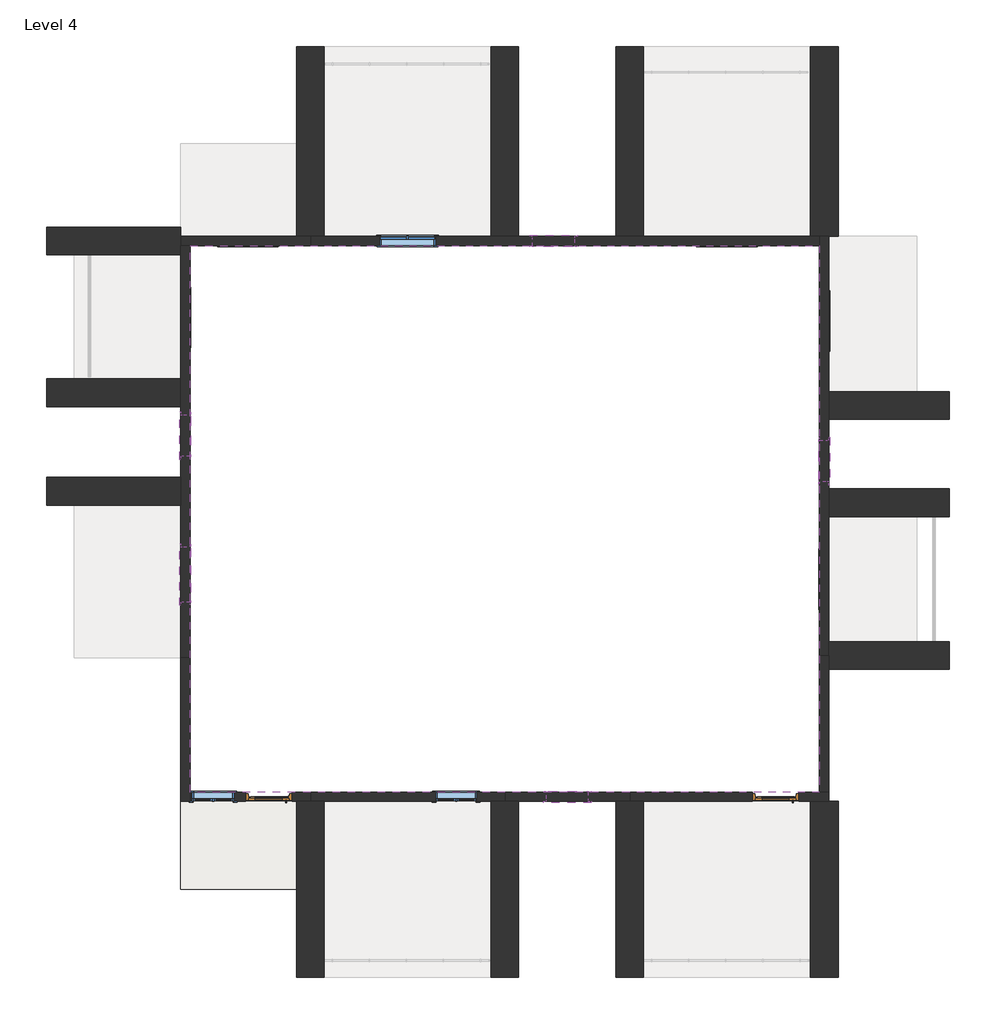
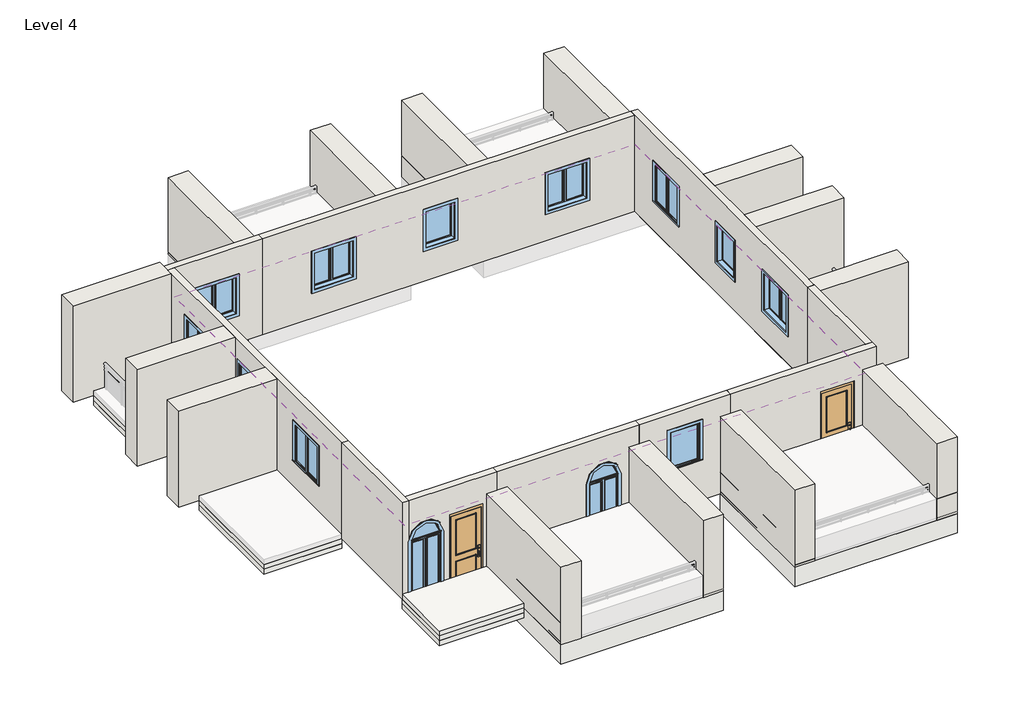
# One storey, part 1 of 2: 24 walls, 13 windows, 5 slabs, 2 doors, 1 covering.
"""IFC4 building model written with IfcOpenShell, lengths in millimetres."""

from ifc_helpers import new_model, si_unit, frame, origin, place, context, project, spatial, polyline, circle_curve, outline, extrude, faceted_brep, transform, mapped, element, save
from ifc_brep_helpers import plane_surface, revolved_surface, advanced_brep
from components import door_b6c2ee01, window_4e95f2a8, window_0862ab64, window_3a1167bf, window_8a4441b2

model = new_model("IFC4")

# Units and contexts
model_context = context("Model", 3, world=origin())
ifc_project = project(units=[si_unit("LENGTHUNIT", "METRE", prefix="MILLI")], contexts=[model_context])

# Site, building, storey
site = spatial("IfcSite", under=ifc_project)
building = spatial("IfcBuilding", under=site)
storey = spatial("IfcBuildingStorey", under=building, Name="Level 4", Elevation=9144.0)

# Covering
placement = place(None, origin())
element("IfcCovering", 1, ObjectType="2' x 4' ACT System", at=placement, inside=storey, context=model_context, shape_type="SweptSolid", body=[
    extrude(outline(polyline([(-12179.4937431, 6319.013611), (-9537.8937431, 6319.013611), (1638.1062569, 6319.013611), (1638.1062569, -2672.586389), (1638.1062569, -5669.786389), (-2527.4937431, -5669.786389), (-5270.6937431, -5669.786389), (-9537.8937431, -5669.786389), (-12179.4937431, -5669.786389), (-12179.4937431, -2723.386389), (-12179.4937431, 6319.013611)])), frame((0.0, 0.0, 11582.4), z_axis=(0.0, 0.0, 1.0), x_axis=(1.0, 0.0, 0.0)), (0.0, 0.0, 1.0), 57.15),
])

# Doors
door_shape = door_b6c2ee01(model_context)
element("IfcDoor", 2, ObjectType="Door-Exterior-Single-Two_Lite : 36\" x 94\"", at=placement, inside=storey, context=model_context, shape_type="MappedRepresentation", body=[
    mapped(door_shape, transform((-10452.2937431, -5765.036389, 9144.0), x_axis=(-1.0, 0.0, 0.0), y_axis=(0.0, -1.0, 0.0), z_axis=(0.0, 0.0, 1.0))),
])
element("IfcDoor", 3, ObjectType="Door-Exterior-Single-Two_Lite : 36\" x 94\"", at=placement, inside=storey, context=model_context, shape_type="MappedRepresentation", body=[
    mapped(door_shape, transform((672.9062569, -5765.036389, 9144.0), x_axis=(-1.0, 0.0, 0.0), y_axis=(0.0, -1.0, 0.0), z_axis=(0.0, 0.0, 1.0))),
])

# Slabs
element("IfcSlab", 4, ObjectType="Generic - 2' 2", at=placement, inside=storey, context=model_context, shape_type="SweptSolid", body=[
    extrude(outline(polyline([(-4965.8937431, -9733.786389), (-9842.6937431, -9733.786389), (-9842.6937431, -5872.986389), (-4965.8937431, -5872.986389), (-4965.8937431, -9733.786389)])), frame((0.0, 0.0, 8839.2), z_axis=(0.0, 0.0, 1.0), x_axis=(1.0, 0.0, 0.0)), (0.0, 0.0, 1.0), 609.6),
])
element("IfcSlab", 5, ObjectType="Generic - 2' 2", at=placement, inside=storey, context=model_context, shape_type="SweptSolid", body=[
    extrude(outline(polyline([(2044.5062569, -9733.786389), (-2832.2937431, -9733.786389), (-2832.2937431, -5872.986389), (2044.5062569, -5872.986389), (2044.5062569, -9733.786389)])), frame((0.0, 0.0, 8839.2), z_axis=(0.0, 0.0, 1.0), x_axis=(1.0, 0.0, 0.0)), (0.0, 0.0, 1.0), 609.6),
])
element("IfcSlab", 6, ObjectType="general 6\"", at=placement, inside=storey, context=model_context, shape_type="SweptSolid", body=[
    extrude(outline(polyline([(-14722.8064179, 6115.813611), (-12382.6937431, 6115.813611), (-12382.6937431, 3398.013611), (-14722.8064179, 3398.013611), (-14722.8064179, 6115.813611)])), frame((0.0, 0.0, 9144.0), z_axis=(0.0, 0.0, 1.0), x_axis=(1.0, 0.0, 0.0)), (0.0, 0.0, 1.0), 152.4),
    extrude(outline(polyline([(-14722.8064179, 629.413611), (-12382.6937431, 629.413611), (-12382.6937431, -2723.386389), (-14722.8064179, -2723.386389), (-14722.8064179, 629.413611)])), frame((0.0, 0.0, 9144.0), z_axis=(0.0, 0.0, 1.0), x_axis=(1.0, 0.0, 0.0)), (0.0, 0.0, 1.0), 152.4),
    extrude(outline(polyline([(-9842.6937431, -5872.986389), (-9842.6937431, -7803.386389), (-12382.6937431, -7803.386389), (-12382.6937431, -5872.986389), (-9842.6937431, -5872.986389)])), frame((0.0, 0.0, 9144.0), z_axis=(0.0, 0.0, 1.0), x_axis=(1.0, 0.0, 0.0)), (0.0, 0.0, 1.0), 152.4),
    extrude(outline(polyline([(3771.7062569, -2367.786389), (1841.3062569, -2367.786389), (1841.3062569, 426.213611), (3771.7062569, 426.213611), (3771.7062569, -2367.786389)])), frame((0.0, 0.0, 9144.0), z_axis=(0.0, 0.0, 1.0), x_axis=(1.0, 0.0, 0.0)), (0.0, 0.0, 1.0), 152.4),
    extrude(outline(polyline([(3771.7062569, 3118.613611), (1841.3062569, 3118.613611), (1841.3062569, 6522.213611), (3771.7062569, 6522.213611), (3771.7062569, 3118.613611)])), frame((0.0, 0.0, 9144.0), z_axis=(0.0, 0.0, 1.0), x_axis=(1.0, 0.0, 0.0)), (0.0, 0.0, 1.0), 152.4),
    extrude(outline(polyline([(-12382.6937431, 6522.213611), (-12382.6937431, 8557.6995084), (-9842.6937431, 8557.6995084), (-9842.6937431, 6522.213611), (-12382.6937431, 6522.213611)])), frame((0.0, 0.0, 9144.0), z_axis=(0.0, 0.0, 1.0), x_axis=(1.0, 0.0, 0.0)), (0.0, 0.0, 1.0), 152.4),
])
element("IfcSlab", 7, ObjectType="general 6\" 2", at=placement, inside=storey, context=model_context, shape_type="SweptSolid", body=[
    extrude(outline(polyline([(3771.7062569, -2367.786389), (1841.3062569, -2367.786389), (1841.3062569, 375.413611), (3771.7062569, 375.413611), (3771.7062569, -2367.786389)])), frame((0.0, 0.0, 9296.4), z_axis=(0.0, 0.0, 1.0), x_axis=(1.0, 0.0, 0.0)), (0.0, 0.0, 1.0), 152.4),
    extrude(outline(polyline([(3771.7062569, 3118.613611), (1841.3062569, 3118.613611), (1841.3062569, 6522.213611), (3771.7062569, 6522.213611), (3771.7062569, 3118.613611)])), frame((0.0, 0.0, 9296.4), z_axis=(0.0, 0.0, 1.0), x_axis=(1.0, 0.0, 0.0)), (0.0, 0.0, 1.0), 152.4),
    extrude(outline(polyline([(-12382.6937431, 6522.213611), (-12382.6937431, 8557.6995084), (-9842.6937431, 8557.6995084), (-9842.6937431, 6522.213611), (-12382.6937431, 6522.213611)])), frame((0.0, 0.0, 9296.4), z_axis=(0.0, 0.0, 1.0), x_axis=(1.0, 0.0, 0.0)), (0.0, 0.0, 1.0), 152.4),
    extrude(outline(polyline([(-14722.8064179, 6115.813611), (-12384.3500805, 6115.813611), (-12384.3500805, 3398.013611), (-14722.8064179, 3398.013611), (-14722.8064179, 6115.813611)])), frame((0.0, 0.0, 9296.4), z_axis=(0.0, 0.0, 1.0), x_axis=(1.0, 0.0, 0.0)), (0.0, 0.0, 1.0), 152.4),
    extrude(outline(polyline([(-14722.8064179, -2723.386389), (-14722.8064179, 629.413611), (-12382.6937431, 629.413611), (-12382.6937431, -2723.386389), (-14722.8064179, -2723.386389)])), frame((0.0, 0.0, 9296.4), z_axis=(0.0, 0.0, 1.0), x_axis=(1.0, 0.0, 0.0)), (0.0, 0.0, 1.0), 152.4),
    extrude(outline(polyline([(-9842.6937431, -5872.986389), (-9842.6937431, -7803.386389), (-12382.6937431, -7803.386389), (-12382.6937431, -5872.986389), (-9842.6937431, -5872.986389)])), frame((0.0, 0.0, 9296.4), z_axis=(0.0, 0.0, 1.0), x_axis=(1.0, 0.0, 0.0)), (0.0, 0.0, 1.0), 152.4),
])
element("IfcSlab", 8, ObjectType="general 6\" 3", at=placement, inside=storey, context=model_context, shape_type="SweptSolid", body=[
    extrude(outline(polyline([(-12382.6937431, -5872.986389), (-9842.6937431, -5872.986389), (-9842.6937431, -7803.386389), (-12382.6937431, -7803.386389), (-12382.6937431, -5872.986389)])), frame((0.0, 0.0, 9448.8), z_axis=(0.0, 0.0, 1.0), x_axis=(1.0, 0.0, 0.0)), (0.0, 0.0, 1.0), 152.4),
])

# Walls
element("IfcWall", 9, ObjectType="Generic - 8\"", at=placement, inside=storey, context=model_context, shape_type="Brep", body=[
    faceted_brep([(-12382.6937431, 6319.013611, 9448.8), (-12179.4937431, 6319.013611, 9448.8), (-9537.8937431, 6319.013611, 9448.8), (-9537.8937431, 6319.013611, 12496.8), (-12179.4937431, 6319.013611, 12496.8), (-12382.6937431, 6319.013611, 12496.8), (-10299.8937431, 6319.013611, 11582.4), (-10299.8937431, 6319.013611, 10363.2), (-11519.0937431, 6319.013611, 10363.2), (-11519.0937431, 6319.013611, 11582.4), (-12382.6937431, 6522.213611, 9448.8), (-12382.6937431, 6522.213611, 12496.8), (-9537.8937431, 6522.213611, 12496.8), (-9537.8937431, 6522.213611, 9448.8), (-9842.6937431, 6522.213611, 9448.8), (-10299.8937431, 6522.213611, 11582.4), (-11519.0937431, 6522.213611, 11582.4), (-11519.0937431, 6522.213611, 10363.2), (-10299.8937431, 6522.213611, 10363.2)], [[[0, 1, 2, 3, 4, 5], [6, 7, 8, 9]], [[10, 11, 12, 13, 14], [15, 16, 17, 18]], [[2, 1, 0, 10, 14, 13]], [[5, 4, 3, 12, 11]], [[0, 5, 11, 10]], [[7, 6, 15, 18]], [[8, 7, 18, 17]], [[9, 8, 17, 16]], [[6, 9, 16, 15]], [[2, 13, 12, 3]]]),
])
element("IfcWall", 10, ObjectType="Generic - 8\"", at=placement, inside=storey, context=model_context, shape_type="Brep", body=[
    faceted_brep([(-12179.4937431, -5872.986389, 9448.8), (-12179.4937431, -5669.786389, 9448.8), (-12179.4937431, -2723.386389, 9448.8), (-12179.4937431, -2723.386389, 12496.8), (-12179.4937431, -5669.786389, 12496.8), (-12179.4937431, -5872.986389, 12496.8), (-12382.6937431, -5872.986389, 9448.8), (-12382.6937431, -5872.986389, 12496.8), (-12382.6937431, -2723.386389, 12496.8), (-12382.6937431, -2723.386389, 9448.8)], [[[0, 1, 2, 3, 4, 5]], [[6, 7, 8, 9]], [[2, 1, 0, 6, 9]], [[3, 2, 9, 8]], [[5, 4, 3, 8, 7]], [[0, 5, 7, 6]]]),
])
element("IfcWall", 11, ObjectType="Generic - 8\"", at=placement, inside=storey, context=model_context, shape_type="Brep", body=[
    faceted_brep([(-2527.4937431, -5669.786389, 12496.8), (1638.1062569, -5669.786389, 12496.8), (1841.3062569, -5669.786389, 12496.8), (1841.3062569, -5669.786389, 9448.8), (1638.1062569, -5669.786389, 9448.8), (1180.9062569, -5669.786389, 9448.8), (1180.9062569, -5669.786389, 11633.2), (164.9062569, -5669.786389, 11633.2), (164.9062569, -5669.786389, 9448.8), (-2527.4937431, -5669.786389, 9448.8), (1841.3062569, -5872.986389, 12496.8), (-2527.4937431, -5872.986389, 12496.8), (-2527.4937431, -5872.986389, 9448.8), (-2222.6937431, -5872.986389, 9448.8), (164.9062569, -5872.986389, 9448.8), (164.9062569, -5872.986389, 11633.2), (1180.9062569, -5872.986389, 11633.2), (1180.9062569, -5872.986389, 9448.8), (1434.9062569, -5872.986389, 9448.8), (1841.3062569, -5872.986389, 9448.8)], [[[0, 1, 2, 3, 4, 5, 6, 7, 8, 9]], [[10, 11, 12, 13, 14, 15, 16, 17, 18, 19]], [[3, 19, 18, 17, 5, 4]], [[12, 9, 8, 14, 13]], [[2, 1, 0, 11, 10]], [[2, 10, 19, 3]], [[7, 15, 14, 8]], [[15, 7, 6, 16]], [[16, 6, 5, 17]], [[9, 12, 11, 0]]]),
])
element("IfcWall", 12, ObjectType="Generic - 8\"", at=placement, inside=storey, context=model_context, shape_type="Brep", body=[
    faceted_brep([(1638.1062569, 6522.213611, 12496.8), (1638.1062569, 6522.213611, 9448.8), (1638.1062569, 6319.013611, 9448.8), (1638.1062569, -2672.586389, 9448.8), (1638.1062569, -2672.586389, 12496.8), (1638.1062569, 6319.013611, 12496.8), (1638.1062569, 1137.413611, 11653.6747769), (1638.1062569, 1137.413611, 10434.4747769), (1638.1062569, 2051.813611, 10434.4747769), (1638.1062569, 2051.813611, 11653.6747769), (1638.1062569, -1605.786389, 11593.5712595), (1638.1062569, -1605.786389, 10374.3712595), (1638.1062569, -386.586389, 10374.3712595), (1638.1062569, -386.586389, 11593.5712595), (1638.1062569, 4058.413611, 11593.5712595), (1638.1062569, 4058.413611, 10374.3712595), (1638.1062569, 5277.613611, 10374.3712595), (1638.1062569, 5277.613611, 11593.5712595), (1841.3062569, 6522.213611, 9448.8), (1841.3062569, 6522.213611, 12496.8), (1841.3062569, 3118.613611, 12496.8), (1841.3062569, 2509.013611, 12496.8), (1841.3062569, 985.013611, 12496.8), (1841.3062569, 375.413611, 12496.8), (1841.3062569, -2367.786389, 12496.8), (1841.3062569, -2672.586389, 12496.8), (1841.3062569, -2672.586389, 9448.8), (1841.3062569, -2367.786389, 9448.8), (1841.3062569, 375.413611, 9448.8), (1841.3062569, 985.013611, 9448.8), (1841.3062569, 2509.013611, 9448.8), (1841.3062569, 3118.613611, 9448.8), (1841.3062569, 1137.413611, 11653.6747769), (1841.3062569, 2051.813611, 11653.6747769), (1841.3062569, 2051.813611, 10434.4747769), (1841.3062569, 1137.413611, 10434.4747769), (1841.3062569, -1605.786389, 11593.5712595), (1841.3062569, -386.586389, 11593.5712595), (1841.3062569, -386.586389, 10374.3712595), (1841.3062569, -1605.786389, 10374.3712595), (1841.3062569, 4058.413611, 11593.5712595), (1841.3062569, 5277.613611, 11593.5712595), (1841.3062569, 5277.613611, 10374.3712595), (1841.3062569, 4058.413611, 10374.3712595)], [[[0, 1, 2, 3, 4, 5], [6, 7, 8, 9], [10, 11, 12, 13], [14, 15, 16, 17]], [[18, 19, 20, 21, 22, 23, 24, 25, 26, 27, 28, 29, 30, 31], [32, 33, 34, 35], [36, 37, 38, 39], [40, 41, 42, 43]], [[3, 2, 1, 18, 31, 30, 29, 28, 27, 26]], [[4, 3, 26, 25]], [[0, 5, 4, 25, 24, 23, 22, 21, 20, 19]], [[0, 19, 18, 1]], [[7, 6, 32, 35]], [[8, 7, 35, 34]], [[9, 8, 34, 33]], [[6, 9, 33, 32]], [[11, 10, 36, 39]], [[12, 11, 39, 38]], [[13, 12, 38, 37]], [[10, 13, 37, 36]], [[15, 14, 40, 43]], [[16, 15, 43, 42]], [[17, 16, 42, 41]], [[14, 17, 41, 40]]]),
])
element("IfcWall", 13, ObjectType="Generic - 8\"", at=placement, inside=storey, context=model_context, shape_type="Brep", body=[
    faceted_brep([(-12179.4937431, -2723.386389, 9448.8), (-12179.4937431, 6319.013611, 9448.8), (-12179.4937431, 6319.013611, 12496.8), (-12179.4937431, -2723.386389, 12496.8), (-12179.4937431, 2610.613611, 11819.7149116), (-12179.4937431, 2610.613611, 10600.5149116), (-12179.4937431, 1696.213611, 10600.5149116), (-12179.4937431, 1696.213611, 11819.7149116), (-12179.4937431, -284.986389, 11642.8059909), (-12179.4937431, -284.986389, 10423.6059909), (-12179.4937431, -1504.186389, 10423.6059909), (-12179.4937431, -1504.186389, 11642.8059909), (-12179.4937431, 5353.813611, 11569.1335827), (-12179.4937431, 5353.813611, 10349.9335827), (-12179.4937431, 4134.613611, 10349.9335827), (-12179.4937431, 4134.613611, 11569.1335827), (-12382.6937431, -2723.386389, 9448.8), (-12382.6937431, -2723.386389, 12496.8), (-12382.6937431, 629.413611, 12496.8), (-12382.6937431, 1239.013611, 12496.8), (-12382.6937431, 2788.413611, 12496.8), (-12382.6937431, 3398.013611, 12496.8), (-12382.6937431, 6115.813611, 12496.8), (-12382.6937431, 6319.013611, 12496.8), (-12382.6937431, 6319.013611, 9448.8), (-12382.6937431, 6115.813611, 9448.8), (-12382.6937431, 3398.013611, 9448.8), (-12382.6937431, 2788.413611, 9448.8), (-12382.6937431, 1239.013611, 9448.8), (-12382.6937431, 629.413611, 9448.8), (-12382.6937431, 2610.613611, 11819.7149116), (-12382.6937431, 1696.213611, 11819.7149116), (-12382.6937431, 1696.213611, 10600.5149116), (-12382.6937431, 2610.613611, 10600.5149116), (-12382.6937431, -284.986389, 11642.8059909), (-12382.6937431, -1504.186389, 11642.8059909), (-12382.6937431, -1504.186389, 10423.6059909), (-12382.6937431, -284.986389, 10423.6059909), (-12382.6937431, 5353.813611, 11569.1335827), (-12382.6937431, 4134.613611, 11569.1335827), (-12382.6937431, 4134.613611, 10349.9335827), (-12382.6937431, 5353.813611, 10349.9335827)], [[[0, 1, 2, 3], [4, 5, 6, 7], [8, 9, 10, 11], [12, 13, 14, 15]], [[16, 17, 18, 19, 20, 21, 22, 23, 24, 25, 26, 27, 28, 29], [30, 31, 32, 33], [34, 35, 36, 37], [38, 39, 40, 41]], [[1, 0, 16, 29, 28, 27, 26, 25, 24]], [[3, 2, 23, 22, 21, 20, 19, 18, 17]], [[0, 3, 17, 16]], [[2, 1, 24, 23]], [[5, 4, 30, 33]], [[6, 5, 33, 32]], [[7, 6, 32, 31]], [[4, 7, 31, 30]], [[9, 8, 34, 37]], [[10, 9, 37, 36]], [[11, 10, 36, 35]], [[8, 11, 35, 34]], [[13, 12, 38, 41]], [[14, 13, 41, 40]], [[15, 14, 40, 39]], [[12, 15, 39, 38]]]),
])
element("IfcWall", 14, ObjectType="Generic - 8\"", at=placement, inside=storey, context=model_context, shape_type="AdvancedBrep", body=[
    advanced_brep(
    [(-12179.4937431, -5669.786389, 12496.8), (-9537.8937431, -5669.786389, 12496.8), (-9537.8937431, -5669.786389, 9448.8), (-9944.2937431, -5669.786389, 9448.8), (-9944.2937431, -5669.786389, 11633.2), (-10960.2937431, -5669.786389, 11633.2), (-10960.2937431, -5669.786389, 9448.8), (-11214.2937431, -5669.786389, 9448.8), (-11214.2937431, -5669.786389, 11187.597687), (-12128.6937431, -5669.786389, 11187.597687), (-12128.6937431, -5669.786389, 9448.8), (-12179.4937431, -5669.786389, 9448.8), (-9537.8937431, -5872.986389, 12496.8), (-12179.4937431, -5872.986389, 12496.8), (-12179.4937431, -5872.986389, 9448.8), (-12128.6937431, -5872.986389, 9448.8), (-12128.6937431, -5872.986389, 11187.597687), (-11214.2937431, -5872.986389, 11187.597687), (-11214.2937431, -5872.986389, 9448.8), (-10960.2937431, -5872.986389, 9448.8), (-10960.2937431, -5872.986389, 11633.2), (-9944.2937431, -5872.986389, 11633.2), (-9944.2937431, -5872.986389, 9448.8), (-9842.6937431, -5872.986389, 9448.8), (-9537.8937431, -5872.986389, 9448.8)],
    [
        (0, 1),
        (1, 2),
        (2, 3),
        (3, 4),
        (4, 5),
        (5, 6),
        (6, 7),
        (7, 8),
        (8, 9, circle_curve(frame((-11671.4937431, -5669.786389, 11187.597687), z_axis=(0.0, -1.0, 0.0), x_axis=(-1.0, 0.0, 0.0)), 457.2)),
        (9, 10),
        (10, 11),
        (11, 0),
        (12, 13),
        (13, 14),
        (14, 15),
        (15, 16),
        (16, 17, circle_curve(frame((-11671.4937431, -5872.986389, 11187.597687), z_axis=(0.0, 1.0, 0.0), x_axis=(-1.0, 0.0, 0.0)), 457.2)),
        (17, 18),
        (18, 19),
        (19, 20),
        (20, 21),
        (21, 22),
        (22, 23),
        (23, 24),
        (24, 12),
        (14, 11),
        (10, 15),
        (2, 24),
        (22, 3),
        (6, 19),
        (18, 7),
        (0, 13),
        (12, 1),
        (5, 20),
        (4, 21),
        (9, 16),
        (17, 8),
    ],
    [
        plane_surface(frame((1423.3958892, -5669.786389, 9448.8), z_axis=(0.0, 1.0, 0.0), x_axis=(-1.0, 0.0, 0.0))),
        plane_surface(frame((1423.3958892, -5872.986389, 9448.8), z_axis=(0.0, -1.0, 0.0), x_axis=(1.0, 0.0, 0.0))),
        plane_surface(frame((-9537.8937431, -5669.786389, 9448.8), z_axis=(0.0, 0.0, -1.0), x_axis=(0.0, -1.0, 0.0))),
        plane_surface(frame((-12281.0937431, -5669.786389, 12496.8), z_axis=(0.0, 0.0, 1.0), x_axis=(0.0, -1.0, 0.0))),
        plane_surface(frame((-12179.4937431, 6416.9740134, 9448.8), z_axis=(-1.0, 0.0, 0.0), x_axis=(0.0, 1.0, 0.0))),
        plane_surface(frame((-9537.8937431, -5669.786389, 12496.8), z_axis=(1.0, 0.0, 0.0), x_axis=(0.0, -1.0, 0.0))),
        plane_surface(frame((-10960.2937431, -4145.786389, 9144.0), z_axis=(1.0, 0.0, 0.0), x_axis=(0.0, -1.0, 0.0))),
        plane_surface(frame((-10960.2937431, -4145.786389, 11633.2), z_axis=(0.0, 0.0, -1.0), x_axis=(0.0, -1.0, 0.0))),
        plane_surface(frame((-9944.2937431, -4145.786389, 11633.2), z_axis=(-1.0, 0.0, 0.0), x_axis=(0.0, -1.0, 0.0))),
        plane_surface(frame((-12128.6937431, -7193.786389, 11187.597687), z_axis=(1.0, 0.0, 0.0), x_axis=(0.0, 1.0, 0.0))),
        plane_surface(frame((-11214.2937431, -7193.786389, 9339.747687), z_axis=(-1.0, 0.0, 0.0), x_axis=(0.0, 1.0, 0.0))),
        revolved_surface(polyline([(-12128.6937431, -5872.986389, 11187.597687), (-12128.6937431, -5669.786389, 11187.597687)]), (-11671.4937431, -4145.786389, 11187.597687), (0.0, -1.0, 0.0)),
    ],
    [
        (0, [[1, 2, 3, 4, 5, 6, 7, 8, 9, 10, 11, 12]]),
        (1, [[13, 14, 15, 16, 17, 18, 19, 20, 21, 22, 23, 24, 25]]),
        (2, [[26, -11, 27, -15]]),
        (2, [[28, -24, -23, 29, -3]]),
        (2, [[30, -19, 31, -7]]),
        (3, [[-1, 32, -13, 33]]),
        (4, [[-12, -26, -14, -32]]),
        (5, [[-33, -25, -28, -2]]),
        (6, [[34, -20, -30, -6]]),
        (7, [[-34, -5, 35, -21]]),
        (8, [[-35, -4, -29, -22]]),
        (9, [[36, -16, -27, -10]]),
        (10, [[37, -8, -31, -18]]),
        (11, [[-36, -9, -37, -17]]),
    ],
),
])
element("IfcWall", 15, ObjectType="Generic - 8\"", at=placement, inside=storey, context=model_context, shape_type="Brep", body=[
    faceted_brep([(1638.1062569, -2672.586389, 9448.8), (1638.1062569, -5669.786389, 9448.8), (1638.1062569, -5669.786389, 12496.8), (1638.1062569, -2672.586389, 12496.8), (1841.3062569, -2672.586389, 9448.8), (1841.3062569, -2672.586389, 12496.8), (1841.3062569, -2977.386389, 12496.8), (1841.3062569, -5669.786389, 12496.8), (1841.3062569, -5669.786389, 9448.8), (1841.3062569, -2977.386389, 9448.8)], [[[0, 1, 2, 3]], [[4, 5, 6, 7, 8, 9]], [[1, 0, 4, 9, 8]], [[3, 2, 7, 6, 5]], [[0, 3, 5, 4]], [[1, 8, 7, 2]]]),
])
element("IfcWall", 16, ObjectType="Generic - 8\"", at=placement, inside=storey, context=model_context, shape_type="Brep", body=[
    faceted_brep([(-9537.8937431, 6319.013611, 12496.8), (-9537.8937431, 6319.013611, 9448.8), (1638.1062569, 6319.013611, 9448.8), (1638.1062569, 6319.013611, 12496.8), (-3746.6937431, 6319.013611, 11680.3983257), (-3746.6937431, 6319.013611, 10461.1983257), (-4661.0937431, 6319.013611, 10461.1983257), (-4661.0937431, 6319.013611, 11680.3983257), (-6794.6937431, 6319.013611, 11529.182989), (-6794.6937431, 6319.013611, 10309.982989), (-8013.8937431, 6319.013611, 10309.982989), (-8013.8937431, 6319.013611, 11529.182989), (215.7062569, 6319.013611, 11566.4159819), (215.7062569, 6319.013611, 10347.2159819), (-1003.4937431, 6319.013611, 10347.2159819), (-1003.4937431, 6319.013611, 11566.4159819), (-9537.8937431, 6522.213611, 9448.8), (-9537.8937431, 6522.213611, 12496.8), (1638.1062569, 6522.213611, 12496.8), (1638.1062569, 6522.213611, 9448.8), (1434.9062569, 6522.213611, 9448.8), (-2222.6937431, 6522.213611, 9448.8), (-2832.2937431, 6522.213611, 9448.8), (-4965.8937431, 6522.213611, 9448.8), (-5575.4937431, 6522.213611, 9448.8), (-9233.0937431, 6522.213611, 9448.8), (-3746.6937431, 6522.213611, 11680.3983257), (-4661.0937431, 6522.213611, 11680.3983257), (-4661.0937431, 6522.213611, 10461.1983257), (-3746.6937431, 6522.213611, 10461.1983257), (-6794.6937431, 6522.213611, 11529.182989), (-8013.8937431, 6522.213611, 11529.182989), (-8013.8937431, 6522.213611, 10309.982989), (-6794.6937431, 6522.213611, 10309.982989), (215.7062569, 6522.213611, 11566.4159819), (-1003.4937431, 6522.213611, 11566.4159819), (-1003.4937431, 6522.213611, 10347.2159819), (215.7062569, 6522.213611, 10347.2159819)], [[[0, 1, 2, 3], [4, 5, 6, 7], [8, 9, 10, 11], [12, 13, 14, 15]], [[16, 17, 18, 19, 20, 21, 22, 23, 24, 25], [26, 27, 28, 29], [30, 31, 32, 33], [34, 35, 36, 37]], [[2, 1, 16, 25, 24, 23, 22, 21, 20, 19]], [[0, 3, 18, 17]], [[2, 19, 18, 3]], [[5, 4, 26, 29]], [[6, 5, 29, 28]], [[7, 6, 28, 27]], [[4, 7, 27, 26]], [[9, 8, 30, 33]], [[10, 9, 33, 32]], [[11, 10, 32, 31]], [[8, 11, 31, 30]], [[13, 12, 34, 37]], [[14, 13, 37, 36]], [[15, 14, 36, 35]], [[12, 15, 35, 34]], [[0, 17, 16, 1]]]),
])
element("IfcWall", 17, ObjectType="Generic - 8\"", at=placement, inside=storey, context=model_context, shape_type="Brep", body=[
    faceted_brep([(-2527.4937431, -5669.786389, 12496.8), (-2527.4937431, -5669.786389, 9448.8), (-5270.6937431, -5669.786389, 9448.8), (-5270.6937431, -5669.786389, 12496.8), (-4356.2937431, -5669.786389, 11943.074951), (-4356.2937431, -5669.786389, 10723.874951), (-3441.8937431, -5669.786389, 10723.874951), (-3441.8937431, -5669.786389, 11943.074951), (-2527.4937431, -5872.986389, 9448.8), (-2527.4937431, -5872.986389, 12496.8), (-5270.6937431, -5872.986389, 12496.8), (-5270.6937431, -5872.986389, 9448.8), (-4965.8937431, -5872.986389, 9448.8), (-2832.2937431, -5872.986389, 9448.8), (-4356.2937431, -5872.986389, 11943.074951), (-3441.8937431, -5872.986389, 11943.074951), (-3441.8937431, -5872.986389, 10723.874951), (-4356.2937431, -5872.986389, 10723.874951)], [[[0, 1, 2, 3], [4, 5, 6, 7]], [[8, 9, 10, 11, 12, 13], [14, 15, 16, 17]], [[2, 1, 8, 13, 12, 11]], [[0, 3, 10, 9]], [[5, 4, 14, 17]], [[6, 5, 17, 16]], [[7, 6, 16, 15]], [[4, 7, 15, 14]], [[0, 9, 8, 1]], [[2, 11, 10, 3]]]),
])
element("IfcWall", 18, ObjectType="Generic - 8\"", at=placement, inside=storey, context=model_context, shape_type="AdvancedBrep", body=[
    advanced_brep(
    [(-9537.8937431, -5669.786389, 12496.8), (-5270.6937431, -5669.786389, 12496.8), (-5270.6937431, -5669.786389, 9448.8), (-5880.2937431, -5669.786389, 9448.8), (-5880.2937431, -5669.786389, 11144.25), (-6794.6937431, -5669.786389, 11144.25), (-6794.6937431, -5669.786389, 9448.8), (-9537.8937431, -5669.786389, 9448.8), (-5270.6937431, -5872.986389, 12496.8), (-9537.8937431, -5872.986389, 12496.8), (-9537.8937431, -5872.986389, 9448.8), (-9233.0937431, -5872.986389, 9448.8), (-6794.6937431, -5872.986389, 9448.8), (-6794.6937431, -5872.986389, 11144.25), (-5880.2937431, -5872.986389, 11144.25), (-5880.2937431, -5872.986389, 9448.8), (-5575.4937431, -5872.986389, 9448.8), (-5270.6937431, -5872.986389, 9448.8)],
    [
        (0, 1),
        (1, 2),
        (2, 3),
        (3, 4),
        (4, 5, circle_curve(frame((-6337.4937431, -5669.786389, 11144.25), z_axis=(0.0, -1.0, 0.0), x_axis=(-1.0, 0.0, 0.0)), 457.2)),
        (5, 6),
        (6, 7),
        (7, 0),
        (8, 9),
        (9, 10),
        (10, 11),
        (11, 12),
        (12, 13),
        (13, 14, circle_curve(frame((-6337.4937431, -5872.986389, 11144.25), z_axis=(0.0, 1.0, 0.0), x_axis=(-1.0, 0.0, 0.0)), 457.2)),
        (14, 15),
        (15, 16),
        (16, 17),
        (17, 8),
        (10, 7),
        (6, 12),
        (2, 17),
        (15, 3),
        (0, 9),
        (8, 1),
        (5, 13),
        (14, 4),
    ],
    [
        plane_surface(frame((1423.3958892, -5669.786389, 9448.8), z_axis=(0.0, 1.0, 0.0), x_axis=(-1.0, 0.0, 0.0))),
        plane_surface(frame((1423.3958892, -5872.986389, 9448.8), z_axis=(0.0, -1.0, 0.0), x_axis=(1.0, 0.0, 0.0))),
        plane_surface(frame((-5270.6937431, -5669.786389, 9448.8), z_axis=(0.0, 0.0, -1.0), x_axis=(0.0, -1.0, 0.0))),
        plane_surface(frame((-9537.8937431, -5669.786389, 12496.8), z_axis=(0.0, 0.0, 1.0), x_axis=(0.0, -1.0, 0.0))),
        plane_surface(frame((-6794.6937431, -7193.786389, 11144.25), z_axis=(1.0, 0.0, 0.0), x_axis=(0.0, 1.0, 0.0))),
        plane_surface(frame((-5880.2937431, -7193.786389, 9296.4), z_axis=(-1.0, 0.0, 0.0), x_axis=(0.0, 1.0, 0.0))),
        revolved_surface(polyline([(-6794.6937431, -5872.986389, 11144.25), (-6794.6937431, -5669.786389, 11144.25)]), (-6337.4937431, -4145.786389, 11144.25), (0.0, -1.0, 0.0)),
        plane_surface(frame((-5270.6937431, -5669.786389, 12496.8), z_axis=(1.0, 0.0, 0.0), x_axis=(0.0, -1.0, 0.0))),
        plane_surface(frame((-9537.8937431, -5669.786389, 9448.8), z_axis=(-1.0, 0.0, 0.0), x_axis=(0.0, -1.0, 0.0))),
    ],
    [
        (0, [[1, 2, 3, 4, 5, 6, 7, 8]]),
        (1, [[9, 10, 11, 12, 13, 14, 15, 16, 17, 18]]),
        (2, [[19, -7, 20, -12, -11]]),
        (2, [[21, -17, -16, 22, -3]]),
        (3, [[-1, 23, -9, 24]]),
        (4, [[25, -13, -20, -6]]),
        (5, [[26, -4, -22, -15]]),
        (6, [[-25, -5, -26, -14]]),
        (7, [[-24, -18, -21, -2]]),
        (8, [[-19, -10, -23, -8]]),
    ],
),
])
element("IfcWall", 19, ObjectType="Generic -2' 2", at=placement, inside=storey, context=model_context, shape_type="Brep", body=[
    faceted_brep([(-12382.6937431, 6725.413611, 9448.8), (-15329.0937431, 6725.413611, 9448.8), (-15329.0937431, 6725.413611, 12496.8), (-12382.6937431, 6725.413611, 12496.8), (-12382.6937431, 6115.813611, 9448.8), (-12382.6937431, 6115.813611, 12496.8), (-15329.0937431, 6115.813611, 12496.8), (-15329.0937431, 6115.813611, 9448.8), (-12382.6937431, 6522.213611, 9448.8), (-12382.6937431, 6319.013611, 9448.8), (-12382.6937431, 6319.013611, 12496.8), (-12382.6937431, 6522.213611, 12496.8)], [[[0, 1, 2, 3]], [[4, 5, 6, 7]], [[1, 0, 8, 9, 4, 7]], [[2, 1, 7, 6]], [[3, 2, 6, 5, 10, 11]], [[0, 3, 11, 10, 5, 4, 9, 8]]]),
])
element("IfcWall", 20, ObjectType="Generic -2' 2", at=placement, inside=storey, context=model_context, shape_type="SweptSolid", body=[
    extrude(outline(polyline([(-15329.0937431, 3398.013611), (-12382.6937431, 3398.013611), (-12382.6937431, 2788.413611), (-15329.0937431, 2788.413611), (-15329.0937431, 3398.013611)])), frame((0.0, 0.0, 9448.8), z_axis=(0.0, 0.0, 1.0), x_axis=(1.0, 0.0, 0.0)), (0.0, 0.0, 1.0), 3048.0),
])
element("IfcWall", 21, ObjectType="Generic -2' 2", at=placement, inside=storey, context=model_context, shape_type="SweptSolid", body=[
    extrude(outline(polyline([(-15329.0937431, 1239.013611), (-12382.6937431, 1239.013611), (-12382.6937431, 629.413611), (-15329.0937431, 629.413611), (-15329.0937431, 1239.013611)])), frame((0.0, 0.0, 9448.8), z_axis=(0.0, 0.0, 1.0), x_axis=(1.0, 0.0, 0.0)), (0.0, 0.0, 1.0), 3048.0),
])
element("IfcWall", 22, ObjectType="Generic -2' 2", at=placement, inside=storey, context=model_context, shape_type="Brep", body=[
    faceted_brep([(1841.3062569, -2977.386389, 9448.8), (4482.9062569, -2977.386389, 9448.8), (4482.9062569, -2977.386389, 12496.8), (1841.3062569, -2977.386389, 12496.8), (1841.3062569, -2367.786389, 9448.8), (1841.3062569, -2367.786389, 12496.8), (4482.9062569, -2367.786389, 12496.8), (4482.9062569, -2367.786389, 9448.8), (1841.3062569, -2672.586389, 9448.8), (1841.3062569, -2672.586389, 12496.8)], [[[0, 1, 2, 3]], [[4, 5, 6, 7]], [[1, 0, 8, 4, 7]], [[2, 1, 7, 6]], [[3, 2, 6, 5, 9]], [[0, 3, 9, 5, 4, 8]]]),
])
element("IfcWall", 23, ObjectType="Generic -2' 2", at=placement, inside=storey, context=model_context, shape_type="SweptSolid", body=[
    extrude(outline(polyline([(4482.9062569, 375.413611), (1841.3062569, 375.413611), (1841.3062569, 985.013611), (4482.9062569, 985.013611), (4482.9062569, 375.413611)])), frame((0.0, 0.0, 9448.8), z_axis=(0.0, 0.0, 1.0), x_axis=(1.0, 0.0, 0.0)), (0.0, 0.0, 1.0), 3048.0),
])
element("IfcWall", 24, ObjectType="Generic -2' 2", at=placement, inside=storey, context=model_context, shape_type="SweptSolid", body=[
    extrude(outline(polyline([(4482.9062569, 2509.013611), (1841.3062569, 2509.013611), (1841.3062569, 3118.613611), (4482.9062569, 3118.613611), (4482.9062569, 2509.013611)])), frame((0.0, 0.0, 9448.8), z_axis=(0.0, 0.0, 1.0), x_axis=(1.0, 0.0, 0.0)), (0.0, 0.0, 1.0), 3048.0),
])
element("IfcWall", 25, ObjectType="Generic -2' 3 red", at=placement, inside=storey, context=model_context, shape_type="Brep", body=[
    faceted_brep([(1434.9062569, -5872.986389, 9448.8), (1434.9062569, -9733.786389, 9448.8), (1434.9062569, -9733.786389, 11887.2), (1434.9062569, -5872.986389, 11887.2), (2044.5062569, -5872.986389, 9448.8), (2044.5062569, -5872.986389, 11887.2), (2044.5062569, -9733.786389, 11887.2), (2044.5062569, -9733.786389, 9448.8), (1841.3062569, -5872.986389, 9448.8)], [[[0, 1, 2, 3]], [[4, 5, 6, 7]], [[1, 0, 8, 4, 7]], [[2, 1, 7, 6]], [[3, 2, 6, 5]], [[0, 3, 5, 4, 8]]]),
])
element("IfcWall", 26, ObjectType="Generic -2' 3 red", at=placement, inside=storey, context=model_context, shape_type="Brep", body=[
    faceted_brep([(-2832.2937431, -5872.986389, 9448.8), (-2832.2937431, -9733.786389, 9448.8), (-2832.2937431, -9733.786389, 11894.8571637), (-2832.2937431, -5872.986389, 11894.8571637), (-2222.6937431, -5872.986389, 9448.8), (-2222.6937431, -5872.986389, 11894.8571637), (-2222.6937431, -9733.786389, 11894.8571637), (-2222.6937431, -9733.786389, 9448.8), (-2527.4937431, -5872.986389, 9448.8)], [[[0, 1, 2, 3]], [[4, 5, 6, 7]], [[1, 0, 8, 4, 7]], [[2, 1, 7, 6]], [[3, 2, 6, 5]], [[0, 3, 5, 4, 8]]]),
])
element("IfcWall", 27, ObjectType="Generic -2' 3 red", at=placement, inside=storey, context=model_context, shape_type="Brep", body=[
    faceted_brep([(-5575.4937431, -5872.986389, 9448.8), (-5575.4937431, -9733.786389, 9448.8), (-5575.4937431, -9733.786389, 11887.2), (-5575.4937431, -5872.986389, 11887.2), (-4965.8937431, -5872.986389, 9448.8), (-4965.8937431, -5872.986389, 11887.2), (-4965.8937431, -9733.786389, 11887.2), (-4965.8937431, -9733.786389, 9448.8), (-5270.6937431, -5872.986389, 9448.8)], [[[0, 1, 2, 3]], [[4, 5, 6, 7]], [[1, 0, 8, 4, 7]], [[2, 1, 7, 6]], [[3, 2, 6, 5]], [[0, 3, 5, 4, 8]]]),
])
element("IfcWall", 28, ObjectType="Generic -2' 3 red", at=placement, inside=storey, context=model_context, shape_type="Brep", body=[
    faceted_brep([(-9842.6937431, -5872.986389, 9448.8), (-9842.6937431, -9733.786389, 9448.8), (-9842.6937431, -9733.786389, 11907.7612992), (-9842.6937431, -5872.986389, 11907.7612992), (-9233.0937431, -5872.986389, 9448.8), (-9233.0937431, -5872.986389, 11907.7612992), (-9233.0937431, -9733.786389, 11907.7612992), (-9233.0937431, -9733.786389, 9448.8), (-9537.8937431, -5872.986389, 9448.8)], [[[0, 1, 2, 3]], [[4, 5, 6, 7]], [[1, 0, 8, 4, 7]], [[2, 1, 7, 6]], [[3, 2, 6, 5]], [[0, 3, 5, 4, 8]]]),
])
element("IfcWall", 29, ObjectType="Generic -2' 3 red", at=placement, inside=storey, context=model_context, shape_type="Brep", body=[
    faceted_brep([(-9233.0937431, 6522.213611, 9448.8), (-9233.0937431, 10687.813611, 9448.8), (-9233.0937431, 10687.813611, 11887.2), (-9233.0937431, 6522.213611, 11887.2), (-9842.6937431, 6522.213611, 9448.8), (-9842.6937431, 6522.213611, 11887.2), (-9842.6937431, 10687.813611, 11887.2), (-9842.6937431, 10687.813611, 9448.8), (-9537.8937431, 6522.213611, 9448.8)], [[[0, 1, 2, 3]], [[4, 5, 6, 7]], [[1, 0, 8, 4, 7]], [[2, 1, 7, 6]], [[3, 2, 6, 5]], [[0, 3, 5, 4, 8]]]),
])
element("IfcWall", 30, ObjectType="Generic -2' 3 red", at=placement, inside=storey, context=model_context, shape_type="SweptSolid", body=[
    extrude(outline(polyline([(-4965.8937431, 10687.813611), (-4965.8937431, 6522.213611), (-5575.4937431, 6522.213611), (-5575.4937431, 10687.813611), (-4965.8937431, 10687.813611)])), frame((0.0, 0.0, 9448.8), z_axis=(0.0, 0.0, 1.0), x_axis=(1.0, 0.0, 0.0)), (0.0, 0.0, 1.0), 2443.0998934),
])
element("IfcWall", 31, ObjectType="Generic -2' 3 red", at=placement, inside=storey, context=model_context, shape_type="SweptSolid", body=[
    extrude(outline(polyline([(-2222.6937431, 10687.813611), (-2222.6937431, 6522.213611), (-2832.2937431, 6522.213611), (-2832.2937431, 10687.813611), (-2222.6937431, 10687.813611)])), frame((0.0, 0.0, 9448.8), z_axis=(0.0, 0.0, 1.0), x_axis=(1.0, 0.0, 0.0)), (0.0, 0.0, 1.0), 2443.7584708),
])
element("IfcWall", 32, ObjectType="Generic -2' 3 red", at=placement, inside=storey, context=model_context, shape_type="Brep", body=[
    faceted_brep([(2044.5062569, 6522.213611, 9448.8), (2044.5062569, 10687.813611, 9448.8), (2044.5062569, 10687.813611, 11887.2), (2044.5062569, 6522.213611, 11887.2), (1434.9062569, 6522.213611, 9448.8), (1434.9062569, 6522.213611, 11887.2), (1434.9062569, 10687.813611, 11887.2), (1434.9062569, 10687.813611, 9448.8), (1841.3062569, 6522.213611, 9448.8), (1638.1062569, 6522.213611, 9448.8)], [[[0, 1, 2, 3]], [[4, 5, 6, 7]], [[1, 0, 8, 9, 4, 7]], [[2, 1, 7, 6]], [[3, 2, 6, 5]], [[0, 3, 5, 4, 9, 8]]]),
])

# Windows
window_shape = window_4e95f2a8(model_context)
element("IfcWindow", 33, ObjectType="36\" x 72\"", at=placement, inside=storey, context=model_context, shape_type="MappedRepresentation", body=[
    mapped(window_shape, transform((-11663.491585, -5771.386389, 9034.947687), x_axis=(-1.0, 0.0, 0.0), y_axis=(0.0, -1.0, 0.0), z_axis=(0.0, 0.0, 1.0))),
])
element("IfcWindow", 34, ObjectType="36\" x 72\"", at=placement, inside=storey, context=model_context, shape_type="MappedRepresentation", body=[
    mapped(window_shape, transform((-6329.491585, -5771.386389, 8991.6), x_axis=(-1.0, 0.0, 0.0), y_axis=(0.0, -1.0, 0.0), z_axis=(0.0, 0.0, 1.0))),
])
window_2_shape = window_0862ab64(model_context)
element("IfcWindow", 35, ObjectType="Casement Dbl with Trim.0001 : 48\" x 48\"", at=placement, inside=storey, context=model_context, shape_type="MappedRepresentation", body=[
    mapped(window_2_shape, transform((-12262.0437431, -894.586389, 9509.2059909), x_axis=(0.0, 1.0, 0.0), y_axis=(-1.0, 0.0, 0.0), z_axis=(0.0, 0.0, 1.0))),
])
element("IfcWindow", 36, ObjectType="Casement Dbl with Trim.0001 : 48\" x 48\"", at=placement, inside=storey, context=model_context, shape_type="MappedRepresentation", body=[
    mapped(window_2_shape, transform((-12262.0437431, 4744.213611, 9435.5335827), x_axis=(0.0, 1.0, 0.0), y_axis=(-1.0, 0.0, 0.0), z_axis=(0.0, 0.0, 1.0))),
])
element("IfcWindow", 37, ObjectType="Casement Dbl with Trim.0001 : 48\" x 48\"", at=placement, inside=storey, context=model_context, shape_type="MappedRepresentation", body=[
    mapped(window_2_shape, transform((-7404.2937431, 6401.563611, 9395.582989), x_axis=(1.0, 0.0, 0.0), y_axis=(0.0, 1.0, 0.0), z_axis=(0.0, 0.0, 1.0))),
])
element("IfcWindow", 38, ObjectType="Casement Dbl with Trim.0001 : 48\" x 48\"", at=placement, inside=storey, context=model_context, shape_type="MappedRepresentation", body=[
    mapped(window_2_shape, transform((-393.8937431, 6401.563611, 9432.8159819), x_axis=(1.0, 0.0, 0.0), y_axis=(0.0, 1.0, 0.0), z_axis=(0.0, 0.0, 1.0))),
])
element("IfcWindow", 39, ObjectType="Casement Dbl with Trim.0001 : 48\" x 48\"", at=placement, inside=storey, context=model_context, shape_type="MappedRepresentation", body=[
    mapped(window_2_shape, transform((1720.6562569, -996.186389, 9459.9712595), x_axis=(0.0, -1.0, 0.0), y_axis=(1.0, 0.0, 0.0), z_axis=(0.0, 0.0, 1.0))),
])
element("IfcWindow", 40, ObjectType="Casement Dbl with Trim.0001 : 48\" x 48\"", at=placement, inside=storey, context=model_context, shape_type="MappedRepresentation", body=[
    mapped(window_2_shape, transform((-10909.4937431, 6401.563611, 9448.8), x_axis=(1.0, 0.0, 0.0), y_axis=(0.0, 1.0, 0.0), z_axis=(0.0, 0.0, 1.0))),
])
window_3_shape = window_3a1167bf(model_context)
element("IfcWindow", 41, ObjectType="Casement Dbl with Trim.0001 : 48\" x 48\"", at=placement, inside=storey, context=model_context, shape_type="MappedRepresentation", body=[
    mapped(window_3_shape, transform((1758.7562569, 4668.013611, 9459.9712595), x_axis=(0.0, -1.0, 0.0), y_axis=(1.0, 0.0, 0.0), z_axis=(0.0, 0.0, 1.0))),
])
window_4_shape = window_8a4441b2(model_context)
element("IfcWindow", 42, ObjectType="Casement with Trim : 36\" x 48\"", at=placement, inside=storey, context=model_context, shape_type="MappedRepresentation", body=[
    mapped(window_4_shape, transform((-3899.0937431, -5771.386389, 9809.474951), x_axis=(-1.0, 0.0, 0.0), y_axis=(0.0, -1.0, 0.0), z_axis=(0.0, 0.0, 1.0))),
])
element("IfcWindow", 43, ObjectType="Casement with Trim : 36\" x 48\"", at=placement, inside=storey, context=model_context, shape_type="MappedRepresentation", body=[
    mapped(window_4_shape, transform((-12281.0937431, 2153.413611, 9686.1149116), x_axis=(0.0, 1.0, 0.0), y_axis=(-1.0, 0.0, 0.0), z_axis=(0.0, 0.0, 1.0))),
])
element("IfcWindow", 44, ObjectType="Casement with Trim : 36\" x 48\"", at=placement, inside=storey, context=model_context, shape_type="MappedRepresentation", body=[
    mapped(window_4_shape, transform((-4203.8937431, 6420.613611, 9546.7983257), x_axis=(1.0, 0.0, 0.0), y_axis=(0.0, 1.0, 0.0), z_axis=(0.0, 0.0, 1.0))),
])
element("IfcWindow", 45, ObjectType="Casement with Trim : 36\" x 48\"", at=placement, inside=storey, context=model_context, shape_type="MappedRepresentation", body=[
    mapped(window_4_shape, transform((1739.7062569, 1594.613611, 9520.0747769), x_axis=(0.0, -1.0, 0.0), y_axis=(1.0, 0.0, 0.0), z_axis=(0.0, 0.0, 1.0))),
])

save(model, "model.ifc")

# Revit data of these elements
# Type "2' x 4' ACT System"
#   Assembly Code = "C3030210"
#   built-in parameter 1002203 = 1 (stored number, unit not read)
#   built-in parameter 1002202 = 1 (stored number, unit not read)
#   Layers, outside or top first: 0' - 1 5/8" "Default" (function 1); 0' - 0 5/8" "Acoustic Ceiling Tile 24 x 48" (function 5)
# Type "Door-Exterior-Single-Two_Lite : 36\" x 94\""
#   Type Mark = "9"
#   Assembly Code = "B2030100"
#   Analytic Construction = "Metal frame, double glass door"
#   Top Rail = 0' - 6"
#   Threshold Offset [instance default] = 0' - 0 1/2"
#   Threshold Length [instance default] = 3' - 4"
#   Thickness = 0' - 1 3/4"
#   Thermal Resistance (R) = 1.3794 (h·ft²·°F)/BTU
#   Swing Angle [instance default] = 90.00°
#   Strike Height = 3' - 4"
#   Stiles = 0' - 6"
#   Rough Width [instance default] = 3' - 4"
#   Rough Height [instance default] = 8' - 2"
#   MFOpeningHeight [instance default] = 0' - 4"
#   MFOpeningWidth [instance default] = 0' - 4"
#   Lock Rail = 0' - 7 1/2"
#   Heat Transfer Coefficient (U) = 0.7250 BTU/(h·ft²·°F)
#   Glass Thickness = 0' - 0 3/4"
#   Inset Calculate [instance default] = 0' - 4"
#   Masonry Inset [instance default] = 0' - 1"
#   Height = 7' - 10"
#   Width = 3' - 0"
#   Masonry Frame Depth = 0' - 5 3/4"
#   Bottom Rail = 0' - 10"
#   Masonry Frame [instance default] = yes
#   Function = 1
#   Threshold [instance default] = yes
#   Dry Wall Frame [instance default] = no
#   Threshold Material = none
#   Panic Bar Material = Metal - Stainless Steel
#   Panel Material = Metal - Painted - Grey
#   Glass Stop Material = Metal - Painted - Grey
#   Exterior Pull Material = Metal - Stainless Steel
#   Frame Material = Metal - Painted - Grey
#   Visual Light Transmittance = 0
#   Solar Heat Gain Coefficient = 0
#   Wall Closure = (empty or 0)
# Type "Generic - 2' 2"
#   Assembly Code = "B1010"
#   Function = 0
#   Layers, outside or top first: 2' - 0" "Damp-proofing" (function 1)
# Type "general 6\""
#   Assembly Code = "B1010"
#   Function = 0
#   Layers, outside or top first: 0' - 6" "Concrete Masonry Units" (function 1)
# Type "general 6\" 2"
#   Assembly Code = "B1010"
#   Function = 0
#   Layers, outside or top first: 0' - 6" "Damp-proofing" (function 1)
# Type "general 6\" 3"
#   Assembly Code = "B1010"
#   Function = 0
#   Layers, outside or top first: 0' - 6" "Door - Frame" (function 1)
# Type "Generic - 8\""
#   Assembly Code = "B2010"
#   Layers, outside or top first: 0' - 8" no material (function 1)
# Type "Generic -2' 2"
#   Assembly Code = "B2010"
#   Layers, outside or top first: 2' - 0" "Damp-proofing" (function 1)
# Type "Generic -2' 3 red"
#   Assembly Code = "B2010"
#   Layers, outside or top first: 2' - 0" "Damp-proofing" (function 1)
# Type "36\" x 72\""
#   Type Mark = "10"
#   Construction Type Id = "SGL"
#   Assembly Code = "B2020100"
#   Analytic Construction = "Large single-glazed windows"
#   Visual Light Transmittance = 0.9
#   Solar Heat Gain Coefficient = 0.86
#   Heat Transfer Coefficient (U) = 0.979472 BTU/(h·ft²·°F)
#   Height = 6' - 0"
#   Default Sill Height = 1' - 0"
#   Trim Projection - Ext. = 0' - 0 1/2"
#   Trim Projection - Int. = 0' - 0 3/4"
#   Trim Width - Exterior = 0' - 3 1/2"
#   Trim Width - Interior = 0' - 3 1/2"
#   Width = 3' - 0"
#   Window Inset = 0' - 0 3/4"
#   Define Thermal Properties by = 1
#   Glass Pane Material = Glass
#   Sash Material = Sash
#   Trim Exterior Material = Trim
#   Trim Interior Material = Trim
#   Wall Closure = (empty or 0)
# Type "Casement Dbl with Trim.0001 : 48\" x 48\""
#   Type Mark = "23"
#   Construction Type Id = "GSP4R"
#   Assembly Code = "B2020100"
#   Analytic Construction = "1/8 in Pilkington single glazing"
#   Visual Light Transmittance = 0.9
#   Solar Heat Gain Coefficient = 0.78
#   Heat Transfer Coefficient (U) = 0.6496 BTU/(h·ft²·°F)
#   Height = 4' - 0"
#   Default Sill Height = 3' - 0"
#   Trim Projection - Ext. = 0' - 0 1/2"
#   Trim Projection - Int. = 0' - 0 3/4"
#   Trim Width - Exterior = 0' - 3 1/2"
#   Trim Width - Interior = 0' - 3 1/2"
#   Width = 4' - 0"
#   Window Inset = 0' - 0 3/4"
#   Define Thermal Properties by = 1
#   Glass Pane Material = Glass
#   Sash Material = Sash
#   Trim Exterior Material = Trim
#   Trim Interior Material = Trim
#   Wall Closure = (empty or 0)
# Type "Casement with Trim : 36\" x 48\""
#   Type Mark = "14"
#   Construction Type Id = "GSP4R"
#   Assembly Code = "B2020100"
#   Analytic Construction = "1/8 in Pilkington single glazing"
#   Visual Light Transmittance = 0.9
#   Solar Heat Gain Coefficient = 0.78
#   Heat Transfer Coefficient (U) = 0.6496 BTU/(h·ft²·°F)
#   Height = 4' - 0"
#   Default Sill Height = 3' - 0"
#   Trim Projection - Ext. = 0' - 0 1/2"
#   Trim Projection - Int. = 0' - 0 3/4"
#   Trim Width - Exterior = 0' - 3 1/2"
#   Trim Width - Interior = 0' - 3 1/2"
#   Width = 3' - 0"
#   Window Inset = 0' - 0 3/4"
#   Define Thermal Properties by = 1
#   Glass Pane Material = Glass
#   Sash Material = Sash
#   Trim Exterior Material = Trim
#   Trim Interior Material = Trim
#   Wall Closure = (empty or 0)
# Element 1 (IfcCovering, "2' x 4' ACT System")
#   Height Offset From Level = 8' - 0"
#   Phase Created = New Construction
#   Materials on its faces: "Acoustic Ceiling Tile 24 x 48", "Default"
# Elements 2, 3 (IfcDoor, "Door-Exterior-Single-Two_Lite : 36\" x 94\"")
#   Threshold Offset = 0' - 0 1/2"
#   Threshold Length = 3' - 4"
#   Swing Angle = 90.00°
#   Rough Width = 3' - 4"
#   Rough Height = 8' - 2"
#   Masonry Inset = 0' - 1"
#   MFOpeningWidth = 0' - 4"
#   MFOpeningHeight = 0' - 4"
#   Inset Calculate = 0' - 4"
#   Threshold = yes
#   Masonry Frame = yes
#   Dry Wall Frame = no
#   Phase Created = New Construction
#   Materials on its faces: "Metal - Painted - Grey", "Metal - Stainless Steel", "Glass"
# Elements 4, 5 (IfcSlab, "Generic - 2' 2")
#   Height Offset From Level = 1' - 0"
#   Phase Created = New Construction
#   Materials on its faces: "Gypsum Wall Board", "Damp-proofing"
# Element 6 (IfcSlab, "general 6\"")
#   built-in parameter 1001955 = 3.14159 (stored number, unit not read)
#   Height Offset From Level = 0' - 6"
#   Phase Created = New Construction
#   Materials on its faces: "Concrete Masonry Units"
# Element 7 (IfcSlab, "general 6\" 2")
#   Height Offset From Level = 1' - 0"
#   Phase Created = New Construction
#   Materials on its faces: "Damp-proofing"
# Element 8 (IfcSlab, "general 6\" 3")
#   built-in parameter 1001955 = 3.14159 (stored number, unit not read)
#   Height Offset From Level = 1' - 6"
#   Phase Created = New Construction
#   Materials on its faces: "Door - Frame"
# Elements 9, 11, 12, 15, 16, 18 (IfcWall, "Generic - 8\"")
#   built-in parameter 1001111 = 1' - 0"
#   Top Offset = 0' - 0"
#   Base Offset = 1' - 0"
#   Unconnected Height = 10' - 0"
#   wall height = 10' - 0"
#   Phase Created = New Construction
#   Base Constraint = Level 4
#   Materials on its faces: "Default Wall", "Tile, Porcelain, 4in", "Parking Stripe"
# Element 10 (IfcWall, "Generic - 8\"")
#   built-in parameter 1001111 = 1' - 0"
#   Top Offset = 0' - 0"
#   Base Offset = 1' - 0"
#   Unconnected Height = 10' - 0"
#   wall height = 10' - 0"
#   Phase Created = New Construction
#   Base Constraint = Level 4
#   Materials on its faces: "Tile, Porcelain, 4in", "Parking Stripe", "Default Wall"
# Elements 13, 17 (IfcWall, "Generic - 8\"")
#   built-in parameter 1001111 = 1' - 0"
#   Top Offset = 0' - 0"
#   Base Offset = 1' - 0"
#   Unconnected Height = 10' - 0"
#   wall height = 10' - 0"
#   Phase Created = New Construction
#   Base Constraint = Level 4
#   Materials on its faces: "Default Wall", "Tile, Porcelain, 4in"
# Element 14 (IfcWall, "Generic - 8\"")
#   built-in parameter 1001111 = 1' - 0"
#   Top Offset = 0' - 0"
#   Base Offset = 1' - 0"
#   Unconnected Height = 10' - 0"
#   wall height = 10' - 0"
#   Phase Created = New Construction
#   Base Constraint = Level 4
#   Materials on its faces: "Default Wall", "Parking Stripe", "Tile, Porcelain, 4in"
# Elements 19, 20, 21, 22, 23, 24 (IfcWall, "Generic -2' 2")
#   built-in parameter 1001111 = 1' - 0"
#   Top Offset = 0' - 0"
#   Base Offset = 1' - 0"
#   Unconnected Height = 10' - 0"
#   wall height = 10' - 0"
#   Phase Created = New Construction
#   Base Constraint = Level 4
#   Materials on its faces: "Gypsum Wall Board", "Damp-proofing"
# Elements 25, 27, 29, 32 (IfcWall, "Generic -2' 3 red")
#   built-in parameter 1001111 = 1' - 0"
#   Top Offset = 0' - 0"
#   Base Offset = 1' - 0"
#   Unconnected Height = 8' - 0"
#   wall height = 8' - 0"
#   Phase Created = New Construction
#   Base Constraint = Level 4
#   Materials on its faces: "Damp-proofing"
# Element 26 (IfcWall, "Generic -2' 3 red")
#   built-in parameter 1001111 = 1' - 0"
#   Top Offset = 0' - 0"
#   Base Offset = 1' - 0"
#   Unconnected Height = 8' - 0.30146"
#   wall height = 8' - 0.30146"
#   Phase Created = New Construction
#   Base Constraint = Level 4
#   Materials on its faces: "Damp-proofing"
# Element 28 (IfcWall, "Generic -2' 3 red")
#   built-in parameter 1001111 = 1' - 0"
#   Top Offset = 0' - 0"
#   Base Offset = 1' - 0"
#   Unconnected Height = 8' - 0.8095"
#   wall height = 8' - 0.8095"
#   Phase Created = New Construction
#   Base Constraint = Level 4
#   Materials on its faces: "Damp-proofing"
# Element 30 (IfcWall, "Generic -2' 3 red")
#   built-in parameter 1001111 = 1' - 0"
#   Top Offset = 0' - 0"
#   Base Offset = 1' - 0"
#   Unconnected Height = 8' - 0.18504"
#   wall height = 8' - 0.18504"
#   Phase Created = New Construction
#   Base Constraint = Level 4
#   Materials on its faces: "Damp-proofing"
# Element 31 (IfcWall, "Generic -2' 3 red")
#   built-in parameter 1001111 = 1' - 0"
#   Top Offset = 0' - 0"
#   Base Offset = 1' - 0"
#   Unconnected Height = 8' - 0.21096"
#   wall height = 8' - 0.21096"
#   Phase Created = New Construction
#   Base Constraint = Level 4
#   Materials on its faces: "Damp-proofing"
# Element 33 (IfcWindow, "36\" x 72\"")
#   Mark = "30"
#   Phase Created = New Construction
#   Materials on its faces: "Sash", "Trim", "Glass"
# Element 34 (IfcWindow, "36\" x 72\"")
#   Mark = "31"
#   Phase Created = New Construction
#   Materials on its faces: "Sash", "Trim", "Glass"
# Element 35 (IfcWindow, "Casement Dbl with Trim.0001 : 48\" x 48\"")
#   Mark = "36"
#   Phase Created = New Construction
#   Materials on its faces: "Sash", "Trim", "Glass"
# Element 36 (IfcWindow, "Casement Dbl with Trim.0001 : 48\" x 48\"")
#   Mark = "37"
#   Phase Created = New Construction
#   Materials on its faces: "Sash", "Trim", "Glass"
# Element 37 (IfcWindow, "Casement Dbl with Trim.0001 : 48\" x 48\"")
#   Mark = "38"
#   Phase Created = New Construction
#   Materials on its faces: "Sash", "Trim", "Glass"
# Element 38 (IfcWindow, "Casement Dbl with Trim.0001 : 48\" x 48\"")
#   Mark = "39"
#   Phase Created = New Construction
#   Materials on its faces: "Sash", "Trim", "Glass"
# Element 39 (IfcWindow, "Casement Dbl with Trim.0001 : 48\" x 48\"")
#   Mark = "40"
#   Phase Created = New Construction
#   Materials on its faces: "Sash", "Trim", "Glass"
# Element 40 (IfcWindow, "Casement Dbl with Trim.0001 : 48\" x 48\"")
#   Mark = "42"
#   Phase Created = New Construction
#   Materials on its faces: "Sash", "Trim", "Glass"
# Element 41 (IfcWindow, "Casement Dbl with Trim.0001 : 48\" x 48\"")
#   Mark = "41"
#   Phase Created = New Construction
#   Materials on its faces: "Sash", "Trim", "Glass"
# Element 42 (IfcWindow, "Casement with Trim : 36\" x 48\"")
#   Mark = "32"
#   Phase Created = New Construction
#   Materials on its faces: "Sash", "Trim", "Glass"
# Element 43 (IfcWindow, "Casement with Trim : 36\" x 48\"")
#   Mark = "33"
#   Phase Created = New Construction
#   Materials on its faces: "Sash", "Trim", "Glass"
# Element 44 (IfcWindow, "Casement with Trim : 36\" x 48\"")
#   Mark = "34"
#   Phase Created = New Construction
#   Materials on its faces: "Sash", "Trim", "Glass"
# Element 45 (IfcWindow, "Casement with Trim : 36\" x 48\"")
#   Mark = "35"
#   Phase Created = New Construction
#   Materials on its faces: "Sash", "Trim", "Glass"
# Materials
#   "Default": colour RGB 127 127 127, transparency 0
#   "Acoustic Ceiling Tile 24 x 48": class "Generic", colour RGB 229 229 229, transparency 0, Description = "Acoustic Ceiling Tile 24 x 48", Cost = 0
#   "Metal - Stainless Steel": class "Metal", colour RGB 247 247 247, transparency 0
#   "Metal - Painted - Grey": class "Paint", colour RGB 104 104 104, transparency 0
#   "Damp-proofing": class "Generic", colour RGB 127 127 127, transparency 0, Description = "Damp-proofing", Cost = 0
#   "Concrete Masonry Units": class "Masonry", colour RGB 227 227 227, transparency 0, Description = "Concrete masonry units", Cost = 0
#   "Door - Frame": colour RGB 118 70 51, transparency 0, Cost = 0
#   "Glass": class "Glass", colour RGB 0 128 192, transparency 0.75, Description = "Soda Lime Glass", Cost = 0
#   "Sash": class "Wood", colour RGB 224 178 126, transparency 0
#   "Trim": class "Wood", colour RGB 224 178 126, transparency 0
#   "Gypsum Wall Board": class "Generic", colour RGB 127 127 127, transparency 0, Description = "Gypsum Wall Board", Cost = 0
#   "Default Wall": colour RGB 128 128 128, transparency 0
#   "Tile, Porcelain, 4in": class "Generic", colour RGB 89 87 158, transparency 0, Description = "Porcelain tile, 4\", white", Cost = 0
#   "Parking Stripe": class "Paint", colour RGB 250 250 91, transparency 0, Cost = 0
